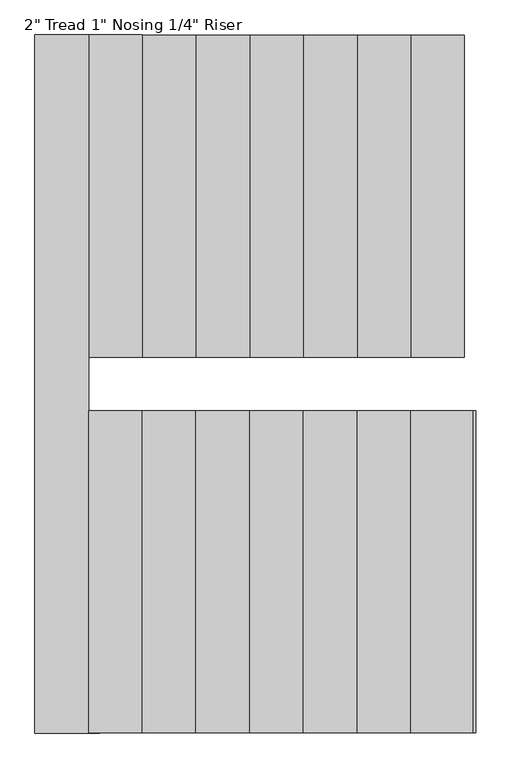
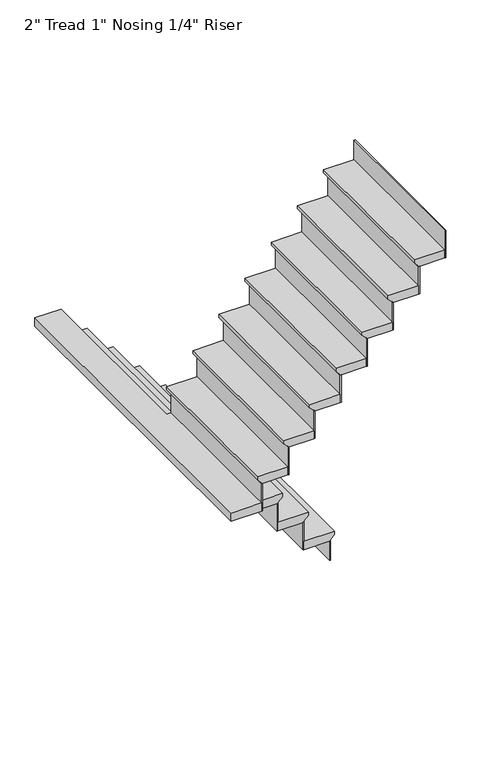
"""IFC4 building model written with IfcOpenShell, lengths in millimetres: stair flight geometry."""

from ifc_helpers import new_model, si_unit, origin, place, context, project, spatial, faceted_brep, source, transform, mapped, element, save


def stair_flight_93877f9a(model_context):
    return source(origin(), model_context, "Body", "Brep", [
        faceted_brep([(3632.2, 10909.3, 12342.2833333), (3632.2, 10909.3, 12361.3333333), (3632.2, 9994.9, 12361.3333333), (3632.2, 9994.9, 12342.2833333), (3606.8, 10909.3, 12316.8833333), (3606.8, 9994.9, 12316.8833333), (3454.4, 10909.3, 12361.3333333), (3454.4, 9994.9, 12361.3333333), (3606.8, 9994.9, 12310.5333333), (3454.4, 9994.9, 12310.5333333), (3454.4, 10909.3, 12310.5333333), (3606.8, 10909.3, 12310.5333333)], [[[0, 1, 2, 3]], [[4, 0, 3, 5]], [[2, 1, 6, 7]], [[8, 9, 10, 11]], [[2, 7, 9, 8, 5, 3]], [[8, 11, 4, 5]], [[6, 1, 0, 4, 11, 10]], [[7, 6, 10, 9]]]),
        faceted_brep([(3606.8, 10909.3, 12310.5333333), (3606.8, 10909.3, 12192.0), (3600.45, 10909.3, 12192.0), (3600.45, 10909.3, 12310.5333333), (3606.8, 9994.9, 12310.5333333), (3600.45, 9994.9, 12310.5333333), (3600.45, 9994.9, 12192.0), (3606.8, 9994.9, 12192.0)], [[[0, 1, 2, 3]], [[4, 5, 6, 7]], [[1, 0, 4, 7]], [[2, 1, 7, 6]], [[3, 2, 6, 5]], [[0, 3, 5, 4]]]),
        faceted_brep([(3454.4, 10909.3, 12479.8666667), (3454.4, 10909.3, 12310.5333333), (3448.05, 10909.3, 12310.5333333), (3448.05, 10909.3, 12479.8666667), (3454.4, 9994.9, 12479.8666667), (3448.05, 9994.9, 12479.8666667), (3448.05, 9994.9, 12310.5333333), (3454.4, 9994.9, 12310.5333333)], [[[0, 1, 2, 3]], [[4, 5, 6, 7]], [[1, 0, 4, 7]], [[2, 1, 7, 6]], [[3, 2, 6, 5]], [[0, 3, 5, 4]]]),
        faceted_brep([(3479.8, 9994.9, 12530.6666667), (3479.8, 10909.3, 12530.6666667), (3302.0, 10909.3, 12530.6666667), (3302.0, 9994.9, 12530.6666667), (3454.4, 9994.9, 12479.8666667), (3302.0, 9994.9, 12479.8666667), (3302.0, 10909.3, 12479.8666667), (3454.4, 10909.3, 12479.8666667), (3454.4, 9994.9, 12486.2166667), (3479.8, 9994.9, 12511.6166667), (3454.4, 10909.3, 12486.2166667), (3479.8, 10909.3, 12511.6166667)], [[[0, 1, 2, 3]], [[4, 5, 6, 7]], [[0, 3, 5, 4, 8, 9]], [[4, 7, 10, 8]], [[2, 1, 11, 10, 7, 6]], [[3, 2, 6, 5]], [[11, 1, 0, 9]], [[10, 11, 9, 8]]]),
        faceted_brep([(3302.0, 10909.3, 12649.2), (3302.0, 10909.3, 12479.8666667), (3295.65, 10909.3, 12479.8666667), (3295.65, 10909.3, 12649.2), (3302.0, 9994.9, 12649.2), (3295.65, 9994.9, 12649.2), (3295.65, 9994.9, 12479.8666667), (3302.0, 9994.9, 12479.8666667)], [[[0, 1, 2, 3]], [[4, 5, 6, 7]], [[1, 0, 4, 7]], [[2, 1, 7, 6]], [[3, 2, 6, 5]], [[0, 3, 5, 4]]]),
        faceted_brep([(3327.4, 9994.9, 12700.0), (3327.4, 10909.3, 12700.0), (3149.6, 10909.3, 12700.0), (3149.6, 9994.9, 12700.0), (3302.0, 9994.9, 12649.2), (3149.6, 9994.9, 12649.2), (3149.6, 10909.3, 12649.2), (3302.0, 10909.3, 12649.2), (3302.0, 9994.9, 12655.55), (3327.4, 9994.9, 12680.95), (3302.0, 10909.3, 12655.55), (3327.4, 10909.3, 12680.95)], [[[0, 1, 2, 3]], [[4, 5, 6, 7]], [[0, 3, 5, 4, 8, 9]], [[4, 7, 10, 8]], [[2, 1, 11, 10, 7, 6]], [[3, 2, 6, 5]], [[11, 1, 0, 9]], [[10, 11, 9, 8]]]),
        faceted_brep([(3149.6, 10909.3, 12818.5333333), (3149.6, 10909.3, 12649.2), (3143.25, 10909.3, 12649.2), (3143.25, 10909.3, 12818.5333333), (3149.6, 9994.9, 12818.5333333), (3143.25, 9994.9, 12818.5333333), (3143.25, 9994.9, 12649.2), (3149.6, 9994.9, 12649.2)], [[[0, 1, 2, 3]], [[4, 5, 6, 7]], [[1, 0, 4, 7]], [[2, 1, 7, 6]], [[3, 2, 6, 5]], [[0, 3, 5, 4]]]),
        faceted_brep([(3175.0, 9994.9, 12869.3333333), (3175.0, 10909.3, 12869.3333333), (2997.2, 10909.3, 12869.3333333), (2997.2, 9994.9, 12869.3333333), (3149.6, 9994.9, 12818.5333333), (2997.2, 9994.9, 12818.5333333), (2997.2, 10909.3, 12818.5333333), (3149.6, 10909.3, 12818.5333333), (3149.6, 9994.9, 12824.8833333), (3175.0, 9994.9, 12850.2833333), (3149.6, 10909.3, 12824.8833333), (3175.0, 10909.3, 12850.2833333)], [[[0, 1, 2, 3]], [[4, 5, 6, 7]], [[0, 3, 5, 4, 8, 9]], [[4, 7, 10, 8]], [[2, 1, 11, 10, 7, 6]], [[3, 2, 6, 5]], [[11, 1, 0, 9]], [[10, 11, 9, 8]]]),
        faceted_brep([(2997.2, 10909.3, 12987.8666667), (2997.2, 10909.3, 12818.5333333), (2990.85, 10909.3, 12818.5333333), (2990.85, 10909.3, 12987.8666667), (2997.2, 9994.9, 12987.8666667), (2990.85, 9994.9, 12987.8666667), (2990.85, 9994.9, 12818.5333333), (2997.2, 9994.9, 12818.5333333)], [[[0, 1, 2, 3]], [[4, 5, 6, 7]], [[1, 0, 4, 7]], [[2, 1, 7, 6]], [[3, 2, 6, 5]], [[0, 3, 5, 4]]]),
        faceted_brep([(3022.6, 9994.9, 13038.6666667), (3022.6, 10909.3, 13038.6666667), (2844.8, 10909.3, 13038.6666667), (2844.8, 9994.9, 13038.6666667), (2997.2, 9994.9, 12987.8666667), (2844.8, 9994.9, 12987.8666667), (2844.8, 10909.3, 12987.8666667), (2997.2, 10909.3, 12987.8666667), (2997.2, 9994.9, 12994.2166667), (3022.6, 9994.9, 13019.6166667), (2997.2, 10909.3, 12994.2166667), (3022.6, 10909.3, 13019.6166667)], [[[0, 1, 2, 3]], [[4, 5, 6, 7]], [[0, 3, 5, 4, 8, 9]], [[4, 7, 10, 8]], [[2, 1, 11, 10, 7, 6]], [[3, 2, 6, 5]], [[11, 1, 0, 9]], [[10, 11, 9, 8]]]),
        faceted_brep([(2844.8, 10909.3, 13157.2), (2844.8, 10909.3, 12987.8666667), (2838.45, 10909.3, 12987.8666667), (2838.45, 10909.3, 13157.2), (2844.8, 9994.9, 13157.2), (2838.45, 9994.9, 13157.2), (2838.45, 9994.9, 12987.8666667), (2844.8, 9994.9, 12987.8666667)], [[[0, 1, 2, 3]], [[4, 5, 6, 7]], [[1, 0, 4, 7]], [[2, 1, 7, 6]], [[3, 2, 6, 5]], [[0, 3, 5, 4]]]),
        faceted_brep([(2870.2, 9994.9, 13208.0), (2870.2, 10909.3, 13208.0), (2692.4, 10909.3, 13208.0), (2692.4, 9994.9, 13208.0), (2844.8, 9994.9, 13157.2), (2692.4, 9994.9, 13157.2), (2692.4, 10909.3, 13157.2), (2844.8, 10909.3, 13157.2), (2844.8, 9994.9, 13163.55), (2870.2, 9994.9, 13188.95), (2844.8, 10909.3, 13163.55), (2870.2, 10909.3, 13188.95)], [[[0, 1, 2, 3]], [[4, 5, 6, 7]], [[0, 3, 5, 4, 8, 9]], [[4, 7, 10, 8]], [[2, 1, 11, 10, 7, 6]], [[3, 2, 6, 5]], [[11, 1, 0, 9]], [[10, 11, 9, 8]]]),
        faceted_brep([(2692.4, 10909.3, 13326.5333333), (2692.4, 10909.3, 13157.2), (2686.05, 10909.3, 13157.2), (2686.05, 10909.3, 13326.5333333), (2692.4, 9994.9, 13326.5333333), (2686.05, 9994.9, 13326.5333333), (2686.05, 9994.9, 13157.2), (2692.4, 9994.9, 13157.2)], [[[0, 1, 2, 3]], [[4, 5, 6, 7]], [[1, 0, 4, 7]], [[2, 1, 7, 6]], [[3, 2, 6, 5]], [[0, 3, 5, 4]]]),
        faceted_brep([(2717.8, 9994.9, 13377.3333333), (2717.8, 10909.3, 13377.3333333), (2540.0, 10909.3, 13377.3333333), (2540.0, 9994.9, 13377.3333333), (2692.4, 9994.9, 13326.5333333), (2540.0, 9994.9, 13326.5333333), (2540.0, 10909.3, 13326.5333333), (2692.4, 10909.3, 13326.5333333), (2692.4, 9994.9, 13332.8833333), (2717.8, 9994.9, 13358.2833333), (2692.4, 10909.3, 13332.8833333), (2717.8, 10909.3, 13358.2833333)], [[[0, 1, 2, 3]], [[4, 5, 6, 7]], [[0, 3, 5, 4, 8, 9]], [[4, 7, 10, 8]], [[2, 1, 11, 10, 7, 6]], [[3, 2, 6, 5]], [[11, 1, 0, 9]], [[10, 11, 9, 8]]]),
        faceted_brep([(2540.0, 10909.3, 13495.8666667), (2540.0, 10909.3, 13326.5333333), (2533.65, 10909.3, 13326.5333333), (2533.65, 10909.3, 13495.8666667), (2540.0, 9994.9, 13495.8666667), (2533.65, 9994.9, 13495.8666667), (2533.65, 9994.9, 13326.5333333), (2540.0, 9994.9, 13326.5333333)], [[[0, 1, 2, 3]], [[4, 5, 6, 7]], [[1, 0, 4, 7]], [[2, 1, 7, 6]], [[3, 2, 6, 5]], [[0, 3, 5, 4]]]),
        faceted_brep([(2590.8, 9842.5, 13546.6666667), (2565.4, 9842.5, 13546.6666667), (2565.4, 10909.3, 13546.6666667), (2413.0, 10909.3, 13546.6666667), (2413.0, 8928.1, 13546.6666667), (2590.8, 8928.1, 13546.6666667), (2565.4, 9842.5, 13495.8666667), (2590.8, 9842.5, 13495.8666667), (2590.8, 8928.1, 13495.8666667), (2413.0, 8928.1, 13495.8666667), (2413.0, 10909.3, 13495.8666667), (2540.0, 10909.3, 13495.8666667), (2540.0, 9994.9, 13495.8666667), (2565.4, 9994.9, 13495.8666667), (2565.4, 9994.9, 13527.6166667), (2565.4, 10909.3, 13527.6166667), (2540.0, 9994.9, 13502.2166667), (2540.0, 10909.3, 13502.2166667)], [[[0, 1, 2, 3, 4, 5]], [[6, 7, 8, 9, 10, 11, 12, 13]], [[1, 0, 7, 6]], [[2, 1, 6, 13, 14, 15]], [[13, 12, 16, 14]], [[12, 11, 17, 16]], [[3, 2, 15, 17, 11, 10]], [[4, 3, 10, 9]], [[5, 4, 9, 8]], [[0, 5, 8, 7]], [[17, 15, 14, 16]]]),
        faceted_brep([(2590.8, 8928.1, 13665.2), (2590.8, 8928.1, 13495.8666667), (2597.15, 8928.1, 13495.8666667), (2597.15, 8928.1, 13665.2), (2590.8, 9842.5, 13665.2), (2597.15, 9842.5, 13665.2), (2597.15, 9842.5, 13495.8666667), (2590.8, 9842.5, 13495.8666667)], [[[0, 1, 2, 3]], [[4, 5, 6, 7]], [[1, 0, 4, 7]], [[2, 1, 7, 6]], [[3, 2, 6, 5]], [[0, 3, 5, 4]]]),
        faceted_brep([(2565.4, 9842.5, 13716.0), (2565.4, 8928.1, 13716.0), (2743.2, 8928.1, 13716.0), (2743.2, 9842.5, 13716.0), (2590.8, 9842.5, 13665.2), (2743.2, 9842.5, 13665.2), (2743.2, 8928.1, 13665.2), (2590.8, 8928.1, 13665.2), (2590.8, 9842.5, 13671.55), (2565.4, 9842.5, 13696.95), (2590.8, 8928.1, 13671.55), (2565.4, 8928.1, 13696.95)], [[[0, 1, 2, 3]], [[4, 5, 6, 7]], [[0, 3, 5, 4, 8, 9]], [[4, 7, 10, 8]], [[2, 1, 11, 10, 7, 6]], [[3, 2, 6, 5]], [[11, 1, 0, 9]], [[10, 11, 9, 8]]]),
        faceted_brep([(2743.2, 8928.1, 13834.5333333), (2743.2, 8928.1, 13665.2), (2749.55, 8928.1, 13665.2), (2749.55, 8928.1, 13834.5333333), (2743.2, 9842.5, 13834.5333333), (2749.55, 9842.5, 13834.5333333), (2749.55, 9842.5, 13665.2), (2743.2, 9842.5, 13665.2)], [[[0, 1, 2, 3]], [[4, 5, 6, 7]], [[1, 0, 4, 7]], [[2, 1, 7, 6]], [[3, 2, 6, 5]], [[0, 3, 5, 4]]]),
        faceted_brep([(2717.8, 9842.5, 13885.3333333), (2717.8, 8928.1, 13885.3333333), (2895.6, 8928.1, 13885.3333333), (2895.6, 9842.5, 13885.3333333), (2743.2, 9842.5, 13834.5333333), (2895.6, 9842.5, 13834.5333333), (2895.6, 8928.1, 13834.5333333), (2743.2, 8928.1, 13834.5333333), (2743.2, 9842.5, 13840.8833333), (2717.8, 9842.5, 13866.2833333), (2743.2, 8928.1, 13840.8833333), (2717.8, 8928.1, 13866.2833333)], [[[0, 1, 2, 3]], [[4, 5, 6, 7]], [[0, 3, 5, 4, 8, 9]], [[4, 7, 10, 8]], [[2, 1, 11, 10, 7, 6]], [[3, 2, 6, 5]], [[11, 1, 0, 9]], [[10, 11, 9, 8]]]),
        faceted_brep([(2895.6, 8928.1, 14003.8666667), (2895.6, 8928.1, 13834.5333333), (2901.95, 8928.1, 13834.5333333), (2901.95, 8928.1, 14003.8666667), (2895.6, 9842.5, 14003.8666667), (2901.95, 9842.5, 14003.8666667), (2901.95, 9842.5, 13834.5333333), (2895.6, 9842.5, 13834.5333333)], [[[0, 1, 2, 3]], [[4, 5, 6, 7]], [[1, 0, 4, 7]], [[2, 1, 7, 6]], [[3, 2, 6, 5]], [[0, 3, 5, 4]]]),
        faceted_brep([(2870.2, 9842.5, 14054.6666667), (2870.2, 8928.1, 14054.6666667), (3048.0, 8928.1, 14054.6666667), (3048.0, 9842.5, 14054.6666667), (2895.6, 9842.5, 14003.8666667), (3048.0, 9842.5, 14003.8666667), (3048.0, 8928.1, 14003.8666667), (2895.6, 8928.1, 14003.8666667), (2895.6, 9842.5, 14010.2166667), (2870.2, 9842.5, 14035.6166667), (2895.6, 8928.1, 14010.2166667), (2870.2, 8928.1, 14035.6166667)], [[[0, 1, 2, 3]], [[4, 5, 6, 7]], [[0, 3, 5, 4, 8, 9]], [[4, 7, 10, 8]], [[2, 1, 11, 10, 7, 6]], [[3, 2, 6, 5]], [[11, 1, 0, 9]], [[10, 11, 9, 8]]]),
        faceted_brep([(3048.0, 8928.1, 14173.2), (3048.0, 8928.1, 14003.8666667), (3054.35, 8928.1, 14003.8666667), (3054.35, 8928.1, 14173.2), (3048.0, 9842.5, 14173.2), (3054.35, 9842.5, 14173.2), (3054.35, 9842.5, 14003.8666667), (3048.0, 9842.5, 14003.8666667)], [[[0, 1, 2, 3]], [[4, 5, 6, 7]], [[1, 0, 4, 7]], [[2, 1, 7, 6]], [[3, 2, 6, 5]], [[0, 3, 5, 4]]]),
        faceted_brep([(3022.6, 9842.5, 14224.0), (3022.6, 8928.1, 14224.0), (3200.4, 8928.1, 14224.0), (3200.4, 9842.5, 14224.0), (3048.0, 9842.5, 14173.2), (3200.4, 9842.5, 14173.2), (3200.4, 8928.1, 14173.2), (3048.0, 8928.1, 14173.2), (3048.0, 9842.5, 14179.55), (3022.6, 9842.5, 14204.95), (3048.0, 8928.1, 14179.55), (3022.6, 8928.1, 14204.95)], [[[0, 1, 2, 3]], [[4, 5, 6, 7]], [[0, 3, 5, 4, 8, 9]], [[4, 7, 10, 8]], [[2, 1, 11, 10, 7, 6]], [[3, 2, 6, 5]], [[11, 1, 0, 9]], [[10, 11, 9, 8]]]),
        faceted_brep([(3200.4, 8928.1, 14342.5333333), (3200.4, 8928.1, 14173.2), (3206.75, 8928.1, 14173.2), (3206.75, 8928.1, 14342.5333333), (3200.4, 9842.5, 14342.5333333), (3206.75, 9842.5, 14342.5333333), (3206.75, 9842.5, 14173.2), (3200.4, 9842.5, 14173.2)], [[[0, 1, 2, 3]], [[4, 5, 6, 7]], [[1, 0, 4, 7]], [[2, 1, 7, 6]], [[3, 2, 6, 5]], [[0, 3, 5, 4]]]),
        faceted_brep([(3175.0, 9842.5, 14393.3333333), (3175.0, 8928.1, 14393.3333333), (3352.8, 8928.1, 14393.3333333), (3352.8, 9842.5, 14393.3333333), (3200.4, 9842.5, 14342.5333333), (3352.8, 9842.5, 14342.5333333), (3352.8, 8928.1, 14342.5333333), (3200.4, 8928.1, 14342.5333333), (3200.4, 9842.5, 14348.8833333), (3175.0, 9842.5, 14374.2833333), (3200.4, 8928.1, 14348.8833333), (3175.0, 8928.1, 14374.2833333)], [[[0, 1, 2, 3]], [[4, 5, 6, 7]], [[0, 3, 5, 4, 8, 9]], [[4, 7, 10, 8]], [[2, 1, 11, 10, 7, 6]], [[3, 2, 6, 5]], [[11, 1, 0, 9]], [[10, 11, 9, 8]]]),
        faceted_brep([(3352.8, 8928.1, 14511.8666667), (3352.8, 8928.1, 14342.5333333), (3359.15, 8928.1, 14342.5333333), (3359.15, 8928.1, 14511.8666667), (3352.8, 9842.5, 14511.8666667), (3359.15, 9842.5, 14511.8666667), (3359.15, 9842.5, 14342.5333333), (3352.8, 9842.5, 14342.5333333)], [[[0, 1, 2, 3]], [[4, 5, 6, 7]], [[1, 0, 4, 7]], [[2, 1, 7, 6]], [[3, 2, 6, 5]], [[0, 3, 5, 4]]]),
        faceted_brep([(3327.4, 9842.5, 14562.6666667), (3327.4, 8928.1, 14562.6666667), (3505.2, 8928.1, 14562.6666667), (3505.2, 9842.5, 14562.6666667), (3352.8, 9842.5, 14511.8666667), (3505.2, 9842.5, 14511.8666667), (3505.2, 8928.1, 14511.8666667), (3352.8, 8928.1, 14511.8666667), (3352.8, 9842.5, 14518.2166667), (3327.4, 9842.5, 14543.6166667), (3352.8, 8928.1, 14518.2166667), (3327.4, 8928.1, 14543.6166667)], [[[0, 1, 2, 3]], [[4, 5, 6, 7]], [[0, 3, 5, 4, 8, 9]], [[4, 7, 10, 8]], [[2, 1, 11, 10, 7, 6]], [[3, 2, 6, 5]], [[11, 1, 0, 9]], [[10, 11, 9, 8]]]),
        faceted_brep([(3505.2, 8928.1, 14681.2), (3505.2, 8928.1, 14511.8666667), (3511.55, 8928.1, 14511.8666667), (3511.55, 8928.1, 14681.2), (3505.2, 9842.5, 14681.2), (3511.55, 9842.5, 14681.2), (3511.55, 9842.5, 14511.8666667), (3505.2, 9842.5, 14511.8666667)], [[[0, 1, 2, 3]], [[4, 5, 6, 7]], [[1, 0, 4, 7]], [[2, 1, 7, 6]], [[3, 2, 6, 5]], [[0, 3, 5, 4]]]),
        faceted_brep([(3657.6, 8928.1, 14850.5333333), (3657.6, 8928.1, 14681.2), (3663.95, 8928.1, 14681.2), (3663.95, 8928.1, 14850.5333333), (3657.6, 9842.5, 14850.5333333), (3663.95, 9842.5, 14850.5333333), (3663.95, 9842.5, 14681.2), (3657.6, 9842.5, 14681.2)], [[[0, 1, 2, 3]], [[4, 5, 6, 7]], [[1, 0, 4, 7]], [[2, 1, 7, 6]], [[3, 2, 6, 5]], [[0, 3, 5, 4]]]),
        faceted_brep([(3479.8, 9842.5, 14732.0), (3479.8, 8928.1, 14732.0), (3657.6, 8928.1, 14732.0), (3657.6, 9842.5, 14732.0), (3505.2, 9842.5, 14681.2), (3657.6, 9842.5, 14681.2), (3657.6, 8928.1, 14681.2), (3505.2, 8928.1, 14681.2), (3505.2, 9842.5, 14687.55), (3479.8, 9842.5, 14712.95), (3505.2, 8928.1, 14687.55), (3479.8, 8928.1, 14712.95)], [[[0, 1, 2, 3]], [[4, 5, 6, 7]], [[0, 3, 5, 4, 8, 9]], [[4, 7, 10, 8]], [[2, 1, 11, 10, 7, 6]], [[3, 2, 6, 5]], [[11, 1, 0, 9]], [[10, 11, 9, 8]]]),
    ])


if __name__ == "__main__":
    model = new_model("IFC4")
    model_context = context("Model", 3, world=origin())
    ifc_project = project(units=[si_unit("LENGTHUNIT", "METRE", prefix="MILLI")], contexts=[model_context])
    site = spatial("IfcSite", under=ifc_project)
    building = spatial("IfcBuilding", under=site)
    placement = place(None, origin())
    stair_flight_shape = stair_flight_93877f9a(model_context)
    element("IfcStairFlight", 1, ObjectType="2\" Tread 1\" Nosing 1/4\" Riser", at=placement, inside=building, context=model_context, shape_type="MappedRepresentation", body=[
        mapped(stair_flight_shape, transform((0.0, 0.0, 0.0), x_axis=(1.0, 0.0, 0.0), y_axis=(0.0, 1.0, 0.0), z_axis=(0.0, 0.0, 1.0))),
    ])
    save(model, "model.ifc")
